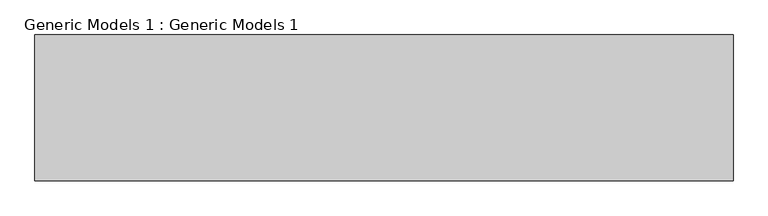
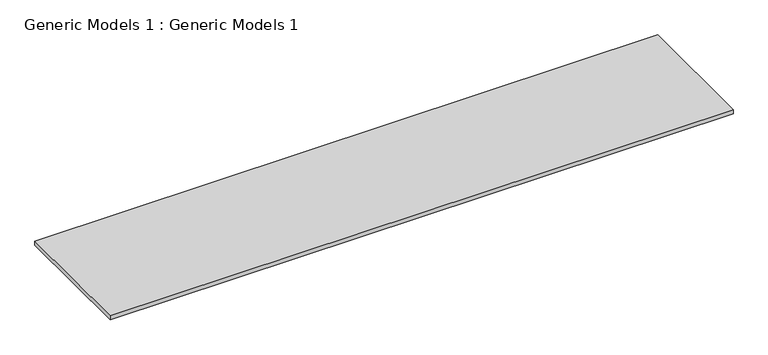
"""IFC4 building model written with IfcOpenShell, lengths in millimetres: proxy geometry, Generic Models 1 : Generic Models 1."""

from ifc_helpers import new_model, si_unit, frame, origin, place, context, project, spatial, polyline, outline, extrude, source, transform, mapped, element, save


def generic_models_1_generic_models_1_de819adb(model_context):
    return source(origin(), model_context, "Body", "SweptSolid", [
        extrude(outline(polyline([(-11453.4088263, -11219.1281855), (11711.3911737, -11219.1281855), (11711.3911737, -16063.1201928), (-11453.4088263, -16063.1201928), (-11453.4088263, -11219.1281855)])), frame((0.0, 0.0, -152.4), z_axis=(0.0, 0.0, 1.0), x_axis=(1.0, 0.0, 0.0)), (0.0, 0.0, 1.0), 152.4),
    ])


if __name__ == "__main__":
    model = new_model("IFC4")
    model_context = context("Model", 3, world=origin())
    ifc_project = project(units=[si_unit("LENGTHUNIT", "METRE", prefix="MILLI")], contexts=[model_context])
    site = spatial("IfcSite", under=ifc_project)
    building = spatial("IfcBuilding", under=site)
    placement = place(None, origin())
    generic_models_1_generic_models_1_shape = generic_models_1_generic_models_1_de819adb(model_context)
    element("IfcBuildingElementProxy", 1, Name="Generic Models 1 : Generic Models 1", ObjectType="Generic Models 1 : Generic Models 1", at=placement, inside=building, context=model_context, shape_type="MappedRepresentation", body=[
        mapped(generic_models_1_generic_models_1_shape, transform((0.0, 0.0, 0.0), x_axis=(1.0, 0.0, 0.0), y_axis=(0.0, 1.0, 0.0), z_axis=(0.0, 0.0, 1.0))),
    ])
    save(model, "model.ifc")
